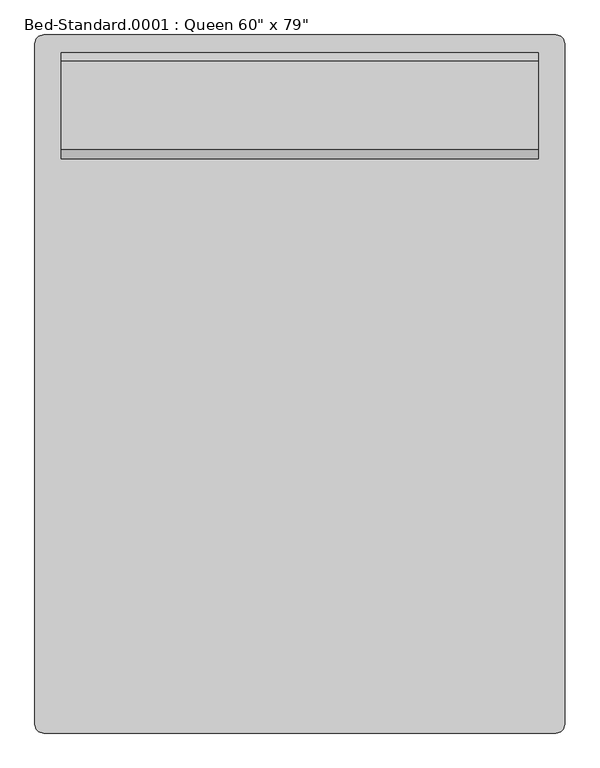
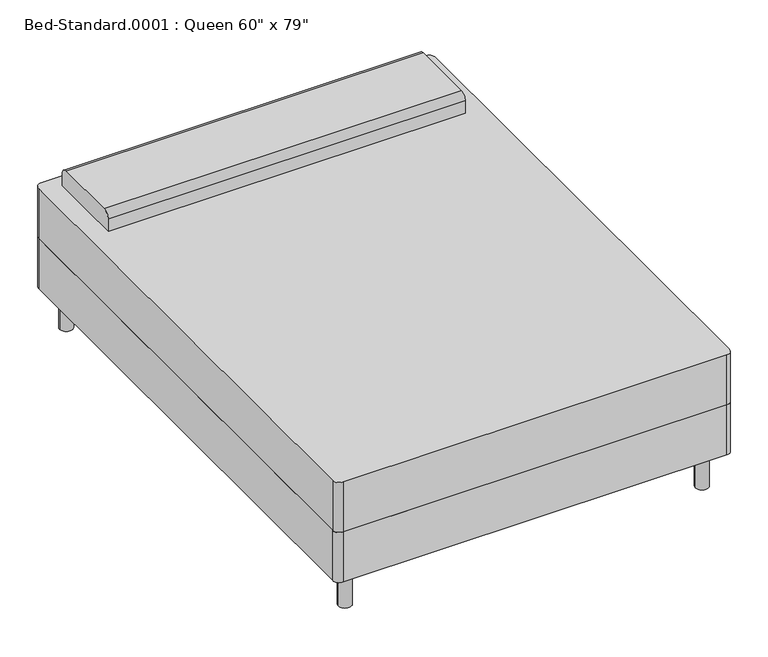
"""IFC4 building model written with IfcOpenShell, lengths in millimetres: furniture geometry."""

from ifc_helpers import new_model, si_unit, point, frame, frame_2d, origin, origin_with_axes, place, context, project, spatial, polyline, circle_curve, trimmed, segment, composite_curve, outline, extrude, source, transform, mapped, element, save


def furniture_e1791683(model_context):
    return source(origin(), model_context, "Body", "SweptSolid", [
        extrude(outline(composite_curve([segment(polyline([(-490.5114754, -1023.495082), (-490.5114754, 932.304918)]), True, "CONTINUOUS"), segment(trimmed(circle_curve(frame_2d((-465.1114754, 932.304918)), 25.4), [point((-490.5114754, 932.304918))], [point((-465.1114754, 957.704918))], False, "CARTESIAN"), True, "CONTINUOUS"), segment(polyline([(-465.1114754, 957.704918), (1008.0885246, 957.704918)]), True, "CONTINUOUS"), segment(trimmed(circle_curve(frame_2d((1008.0885246, 932.304918)), 25.4), [point((1008.0885246, 957.704918))], [point((1033.4885246, 932.304918))], False, "CARTESIAN"), True, "CONTINUOUS"), segment(polyline([(1033.4885246, 932.304918), (1033.4885246, -1023.495082)]), True, "CONTINUOUS"), segment(trimmed(circle_curve(frame_2d((1008.0885246, -1023.495082)), 25.4), [point((1033.4885246, -1023.495082))], [point((1008.0885246, -1048.895082))], False, "CARTESIAN"), True, "CONTINUOUS"), segment(polyline([(1008.0885246, -1048.895082), (-465.1114754, -1048.895082)]), True, "CONTINUOUS"), segment(trimmed(circle_curve(frame_2d((-465.1114754, -1023.495082)), 25.4), [point((-465.1114754, -1048.895082))], [point((-490.5114754, -1023.495082))], False, "CARTESIAN"), True, "CONTINUOUS")], self_intersect=False)), frame((0.0, 0.0, 152.4), z_axis=(0.0, 0.0, 1.0), x_axis=(1.0, 0.0, 0.0)), (0.0, 0.0, 1.0), 203.2),
        extrude(outline(composite_curve([segment(polyline([(602.104918, 558.8), (602.104918, 609.6)]), True, "CONTINUOUS"), segment(trimmed(circle_curve(frame_2d((627.504918, 609.6)), 25.4), [point((602.104918, 609.6))], [point((627.504918, 635.0))], False, "CARTESIAN"), True, "CONTINUOUS"), segment(polyline([(627.504918, 635.0), (881.504918, 635.0)]), True, "CONTINUOUS"), segment(trimmed(circle_curve(frame_2d((881.504918, 609.6)), 25.4), [point((881.504918, 635.0))], [point((906.904918, 609.6))], False, "CARTESIAN"), True, "CONTINUOUS"), segment(polyline([(906.904918, 609.6), (906.904918, 558.8), (602.104918, 558.8)]), True, "CONTINUOUS")], self_intersect=False)), frame((-414.3114754, 0.0, 0.0), z_axis=(1.0, 0.0, 0.0), x_axis=(0.0, 1.0, 0.0)), (0.0, 0.0, 1.0), 1371.6),
        extrude(outline(composite_curve([segment(trimmed(circle_curve(frame_2d((-414.3114754, 881.504918)), 25.4), [point((-439.7114754, 881.504918))], [point((-388.9114754, 881.504918))], False, "CARTESIAN"), True, "CONTINUOUS"), segment(trimmed(circle_curve(frame_2d((-414.3114754, 881.504918)), 25.4), [point((-388.9114754, 881.504918))], [point((-439.7114754, 881.504918))], False, "CARTESIAN"), True, "CONTINUOUS")], self_intersect=False)), origin_with_axes(), (0.0, 0.0, 1.0), 152.4),
        extrude(outline(composite_curve([segment(trimmed(circle_curve(frame_2d((957.2885246, 881.504918)), 25.4), [point((931.8885246, 881.504918))], [point((982.6885246, 881.504918))], False, "CARTESIAN"), True, "CONTINUOUS"), segment(trimmed(circle_curve(frame_2d((957.2885246, 881.504918)), 25.4), [point((982.6885246, 881.504918))], [point((931.8885246, 881.504918))], False, "CARTESIAN"), True, "CONTINUOUS")], self_intersect=False)), origin_with_axes(), (0.0, 0.0, 1.0), 152.4),
        extrude(outline(composite_curve([segment(trimmed(circle_curve(frame_2d((957.2885246, -972.695082)), 25.4), [point((931.8885246, -972.695082))], [point((982.6885246, -972.695082))], False, "CARTESIAN"), True, "CONTINUOUS"), segment(trimmed(circle_curve(frame_2d((957.2885246, -972.695082)), 25.4), [point((982.6885246, -972.695082))], [point((931.8885246, -972.695082))], False, "CARTESIAN"), True, "CONTINUOUS")], self_intersect=False)), origin_with_axes(), (0.0, 0.0, 1.0), 152.4),
        extrude(outline(composite_curve([segment(trimmed(circle_curve(frame_2d((-414.3114754, -972.695082)), 25.4), [point((-439.7114754, -972.695082))], [point((-388.9114754, -972.695082))], False, "CARTESIAN"), True, "CONTINUOUS"), segment(trimmed(circle_curve(frame_2d((-414.3114754, -972.695082)), 25.4), [point((-388.9114754, -972.695082))], [point((-439.7114754, -972.695082))], False, "CARTESIAN"), True, "CONTINUOUS")], self_intersect=False)), origin_with_axes(), (0.0, 0.0, 1.0), 152.4),
        extrude(outline(composite_curve([segment(polyline([(-465.1114754, 957.704918), (1008.0885246, 957.704918)]), True, "CONTINUOUS"), segment(trimmed(circle_curve(frame_2d((1008.0885246, 932.304918)), 25.4), [point((1008.0885246, 957.704918))], [point((1033.4885246, 932.304918))], False, "CARTESIAN"), True, "CONTINUOUS"), segment(polyline([(1033.4885246, 932.304918), (1033.4885246, -1023.495082)]), True, "CONTINUOUS"), segment(trimmed(circle_curve(frame_2d((1008.0885246, -1023.495082)), 25.4), [point((1033.4885246, -1023.495082))], [point((1008.0885246, -1048.895082))], False, "CARTESIAN"), True, "CONTINUOUS"), segment(polyline([(1008.0885246, -1048.895082), (-465.1114754, -1048.895082)]), True, "CONTINUOUS"), segment(trimmed(circle_curve(frame_2d((-465.1114754, -1023.495082)), 25.4), [point((-465.1114754, -1048.895082))], [point((-490.5114754, -1023.495082))], False, "CARTESIAN"), True, "CONTINUOUS"), segment(polyline([(-490.5114754, -1023.495082), (-490.5114754, 932.304918)]), True, "CONTINUOUS"), segment(trimmed(circle_curve(frame_2d((-465.1114754, 932.304918)), 25.4), [point((-490.5114754, 932.304918))], [point((-465.1114754, 957.704918))], False, "CARTESIAN"), True, "CONTINUOUS")], self_intersect=False)), frame((0.0, 0.0, 355.6), z_axis=(0.0, 0.0, 1.0), x_axis=(1.0, 0.0, 0.0)), (0.0, 0.0, 1.0), 203.2),
    ])


if __name__ == "__main__":
    model = new_model("IFC4")
    model_context = context("Model", 3, world=origin())
    ifc_project = project(units=[si_unit("LENGTHUNIT", "METRE", prefix="MILLI")], contexts=[model_context])
    site = spatial("IfcSite", under=ifc_project)
    building = spatial("IfcBuilding", under=site)
    placement = place(None, origin())
    furniture_shape = furniture_e1791683(model_context)
    element("IfcFurniture", 1, ObjectType="Bed-Standard.0001 : Queen 60\" x 79\"", at=placement, inside=building, context=model_context, shape_type="MappedRepresentation", body=[
        mapped(furniture_shape, transform((0.0, 0.0, 0.0), x_axis=(1.0, 0.0, 0.0), y_axis=(0.0, 1.0, 0.0), z_axis=(0.0, 0.0, 1.0))),
    ])
    save(model, "model.ifc")

# Revit data of these elements
# Type "Bed-Standard.0001 : Queen 60\" x 79\""
#   Assembly Code = "E2020200"
#   Length = 6' - 7"
#   Width = 5' - 0"
#   Leg Material = Steel, Chrome Plated
#   Mattress Material = Pine
#   Default Elevation = 0
# Element 1 (IfcFurniture, "Bed-Standard.0001 : Queen 60\" x 79\"")
#   Materials on its faces: "Linen, White", "Steel, Chrome Plated"
# Materials
#   "Steel, Chrome Plated": class "Metal", colour RGB 17 17 17, transparency 0, Description = "Chromiuim plated steel", Cost = 0
#   "Pine": class "Wood", colour RGB 223 192 134, transparency 0, Description = "Pinus Echinata", Cost = 0
#   "Linen, White": class "Textile", colour RGB 247 247 239, transparency 0, Description = "Linen, white", Cost = 0
